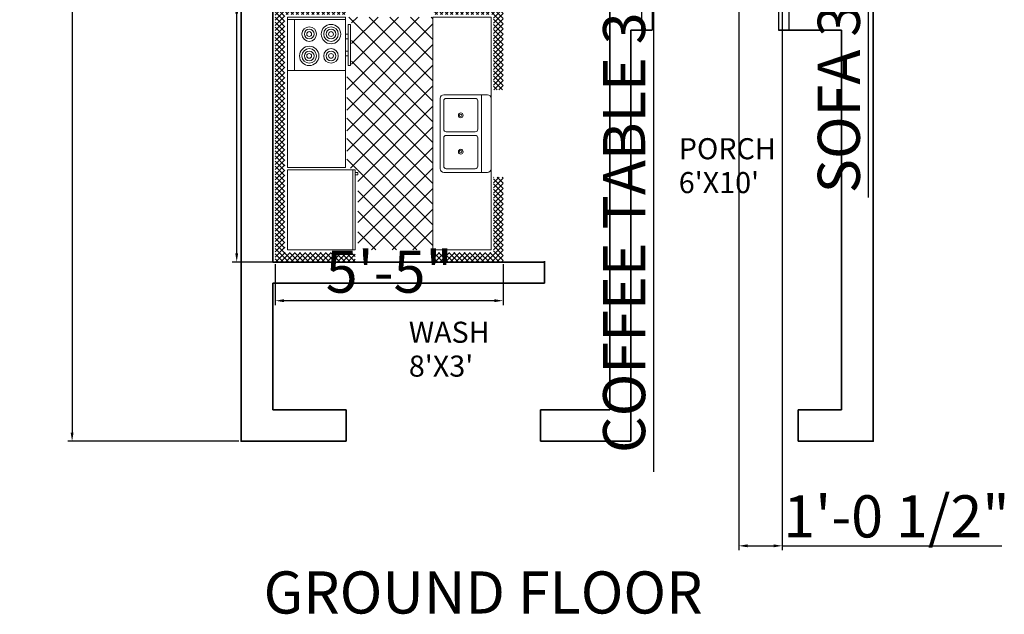
# Model space of a CAD drawing. Units: inches. Extents: x 2353 to 2961, y 642 to 1248.
# Tile 1 of 5: x 2353 to 2633, y 671 to 840. Entities that reach past the tile are written whole.
import ezdxf

# ---------------------------------------------------------------- set-up
doc = ezdxf.new("R2010")
doc.units = ezdxf.units.IN
for name, color, linetype, lineweight in [('A-ANNO-DIMS', 2, 'Continuous', 18), ('A-ANNO-TEXT', 7, 'Continuous', 25), ('A-AREA-IDEN', 7, 'Continuous', 18), ('A-DOOR', 4, 'Continuous', 25), ('A-FLOR-FIXT', 9, 'Continuous', 18), ('A-WALL', 7, 'Continuous', 35)]:
    doc.layers.add(name, color=color, linetype=linetype, lineweight=lineweight)
doc.styles.get("Standard").update_dxf_attribs({"font": 'arial.ttf'})
doc.dimstyles.new('ISO-25', dxfattribs={"dimtxt": 12, "dimasz": 2.5, "dimexe": 1.25, "dimexo": 0.625, "dimtad": 1, "dimdec": 1, "dimlunit": 3, "dimtxsty": 'Standard', "dimcen": 2.5, "dimadec": 0, "dimazin": 0, "dimtfac": 1, "dimtdec": 1, "dimtmove": 0, "dimatfit": 3, "dimfxl": 1, "dimarcsym": 0})

# ---------------------------------------------------------------- blocks, each defined once
blk = doc.blocks.new('Kitchen Layout - 7 x 8 ft')
for p, q in [((-5, 81.32), (2.68, 89)), ((-5, 83.44), (0.56, 89)), ((-5, 85.56), (-1.56, 89)), ((-5, 87.68), (-3.68, 89)), ((-1, 84.97), (-5, 88.97)), ((-1, 82.85), (-5, 86.85)), ((1.09, 85), (-2.91, 89)), ((3.21, 85), (-0.79, 89)), ((0.81, 85), (4.81, 89)), ((5.34, 85), (1.34, 89)), ((2.93, 85), (6.93, 89)), ((7.46, 85), (3.46, 89)), ((5.05, 85), (9.05, 89)), ((9.58, 85), (5.58, 89)), ((7.17, 85), (11.17, 89)), ((11.7, 85), (7.7, 89)), ((9.29, 85), (13.29, 89)), ((13.82, 85), (9.82, 89)), ((11.41, 85), (15.41, 89)), ((15.94, 85), (11.94, 89)), ((13.53, 85), (17.53, 89)), ((18.06, 85), (14.06, 89)), ((15.65, 85), (19.65, 89)), ((20.18, 85), (16.18, 89)), ((17.78, 85), (21.78, 89)), ((22.31, 85), (18.31, 89)), ((19.9, 85), (23.9, 89)), ((24.43, 85), (20.43, 89)), ((22.02, 85), (26.02, 89)), ((26.55, 85), (22.55, 89)), ((24.14, 85), (28.14, 89)), ((28.67, 85), (24.67, 89)), ((26.26, 85), (30.26, 89)), ((30.79, 85), (26.79, 89)), ((28.38, 85), (32.38, 89)), ((32.91, 85), (28.91, 89)), ((30.5, 85), (34.5, 89)), ((35.03, 85), (31.03, 89)), ((32.63, 85), (36.63, 89)), ((37.16, 85), (33.16, 89)), ((34.75, 85), (38.75, 89)), ((39.28, 85), (35.28, 89)), ((36.87, 85), (40.87, 89)), ((41.4, 85), (37.4, 89)), ((38.99, 85), (42.99, 89)), ((43.52, 85), (39.52, 89)), ((41.11, 85), (45.11, 89)), ((45.64, 85), (41.64, 89)), ((43.23, 85), (47.23, 89)), ((47.76, 85), (43.76, 89)), ((45.35, 85), (49.35, 89)), ((49.88, 85), (45.88, 89)), ((47.47, 85), (51.47, 89)), ((52, 85), (48, 89)), ((49.6, 85), (53.6, 89)), ((54.13, 85), (50.13, 89)), ((51.72, 85), (55.72, 89)), ((56.25, 85), (52.25, 89)), ((53.84, 85), (57.84, 89)), ((58.37, 85), (54.37, 89)), ((55.96, 85), (59.96, 89)), ((60.49, 85), (56.49, 89)), ((58.08, 85), (62.08, 89)), ((62.61, 85), (58.61, 89)), ((60.2, 85), (64.2, 89)), ((64.73, 85), (60.73, 89)), ((62.32, 85), (66.32, 89)), ((66.85, 85), (62.85, 89)), ((64.45, 85), (68.45, 89)), ((68.97, 85), (64.97, 89)), ((66.57, 85), (70.57, 89)), ((71.1, 85), (67.1, 89)), ((68.69, 85), (72.69, 89)), ((73.22, 85), (69.22, 89)), ((70.81, 85), (74.81, 89)), ((75.34, 85), (71.34, 89)), ((72.93, 85), (76.93, 89)), ((77.46, 85), (73.46, 89)), ((75.05, 85), (79.05, 89)), ((79.58, 85), (75.58, 89)), ((77.17, 85), (81.17, 89)), ((81.7, 85), (77.7, 89)), ((79.29, 85), (83.29, 89)), ((83.82, 85), (79.82, 89)), ((81.42, 85), (85.42, 89)), ((85.95, 85), (81.95, 89)), ((83.54, 85), (87.54, 89)), ((88.07, 85), (84.07, 89)), ((85.66, 85), (89.66, 89)), ((90.19, 85), (86.19, 89)), ((87.78, 85), (91.78, 89)), ((92.31, 85), (88.31, 89)), ((89.9, 85), (93.9, 89)), ((94.43, 85), (90.43, 89)), ((92.02, 85), (96.02, 89)), ((96.55, 85), (92.55, 89)), ((94.14, 85), (98.14, 89)), ((101, 82.67), (94.67, 89)), ((96.27, 85), (100.27, 89)), ((101, 84.79), (96.79, 89)), ((97, 83.61), (101, 87.61)), ((97, 81.49), (101, 85.49)), ((101, 86.92), (98.92, 89)), ((-1, 80.73), (-5, 84.73)), ((-5, 79.19), (-1, 83.19)), ((-1, 78.61), (-5, 82.61)), ((34, 84), (96, 84)), ((34, 60), (34, 84)), ((96, 84), (96, 60)), ((101, 80.55), (97, 84.55)), ((97, 79.37), (101, 83.37)), ((101, 78.43), (97, 82.43)), ((97, 77.25), (101, 81.25)), ((-5, 77.07), (-1, 81.07)), ((-1, 76.49), (-5, 80.49)), ((-5, 74.95), (-1, 78.95)), ((-1, 74.36), (-5, 78.36)), ((74, 81), (95, 81)), ((101, 76.31), (97, 80.31)), ((97, 75.13), (101, 79.13)), ((101, 74.19), (97, 78.19)), ((-5, 72.83), (-1, 76.83)), ((-1, 72.24), (-5, 76.24)), ((-5, 70.71), (-1, 74.71)), ((-1, 70.12), (-5, 74.12)), ((97, 73.01), (101, 77.01)), ((101, 72.07), (97, 76.07)), ((97, 70.89), (101, 74.89)), ((101, 69.95), (97, 73.95)), ((-5, 68.59), (-1, 72.59)), ((-1, 68), (-5, 72)), ((-5, 66.47), (-1, 70.47)), ((-1, 65.88), (-5, 69.88)), ((97, 68.76), (101, 72.76)), ((101, 67.82), (97, 71.82)), ((97, 66.64), (101, 70.64)), ((101, 65.7), (97, 69.7)), ((-5, 64.35), (-1, 68.35)), ((-1, 63.76), (-5, 67.76)), ((-5, 62.22), (-1, 66.22)), ((-1, 61.64), (-5, 65.64)), ((97, 64.52), (101, 68.52)), ((101, 63.58), (97, 67.58)), ((97, 62.4), (101, 66.4)), ((101, 61.46), (97, 65.46)), ((-5, 60.1), (-1, 64.1)), ((-1, 59.52), (-5, 63.52)), ((-5, 57.98), (-1, 61.98)), ((-1, 57.39), (-5, 61.39)), ((97, 60.28), (101, 64.28)), ((100.34, 60), (97, 63.34)), ((98.22, 60), (97, 61.22)), ((98.84, 60), (101, 62.16)), ((-1.73, 56), (-5, 59.27)), ((-3.85, 56), (-5, 57.15)), ((-4.86, 56), (-1, 59.86)), ((-2.74, 56), (-1, 57.74)), ((0, 57), (33, 57)), ((10.4, 24), (45.9, 59.5)), ((18.88, 24), (54.38, 59.5)), ((27.37, 24), (62.87, 59.5)), ((33.03, 55.11), (37.41, 59.5)), ((67.71, 24), (33.68, 58.04)), ((96, 60), (34, 60)), ((35.85, 24), (71.35, 59.5)), ((76.2, 24), (40.7, 59.5)), ((44.34, 24), (77.84, 57.5)), ((84.68, 24), (49.18, 59.5)), ((52.82, 24), (86.32, 57.5)), ((93.17, 24), (57.67, 59.5)), ((61.31, 24), (96, 58.69)), ((96, 29.65), (66.15, 59.5)), ((96, 38.14), (76.64, 57.5)), ((80, 60), (80, 59)), ((82, 59), (82, 60)), ((96, 46.63), (85.13, 57.5)), ((87, 59), (87, 60)), ((89, 60), (89, 59)), ((96, 55.11), (93.57, 57.54)), ((100.96, 60), (101, 60.04)), ((0, 30.57), (24.43, 55)), ((0, 39.06), (15.94, 55)), ((0, 47.54), (7.46, 55)), ((1.91, 24), (32.91, 55)), ((33.77, 24), (2.77, 55)), ((42.26, 24), (11.26, 55)), ((50.74, 24), (19.74, 55)), ((59.23, 24), (28.23, 55)), ((31, 55), (31, 56)), ((32, 55), (31, 55)), ((32, 56), (32, 55)), ((25.29, 24), (0, 49.29)), ((69.79, 24), (96, 50.21)), ((16.8, 24), (0, 40.8)), ((78.28, 24), (96, 41.72)), ((86.76, 24), (96, 33.24)), ((8.32, 24), (0, 32.32)), ((95.25, 24), (96, 24.75)), ((-5, 21.92), (-2.92, 24)), ((-5, 19.8), (-1, 23.8)), ((-1, 19.21), (-5, 23.21)), ((-5, 17.68), (-1, 21.68)), ((-1, 17.09), (-5, 21.09)), ((-1, 21.33), (-3.67, 24)), ((-1, 23.45), (-1.55, 24)), ((0, 24), (96, 24)), ((0, 0), (0, 24)), ((96, 24), (96, 0)), ((97, 22.1), (98.9, 24)), ((97, 19.97), (101, 23.97)), ((101, 19.03), (97, 23.03)), ((97, 17.85), (101, 21.85)), ((101, 16.91), (97, 20.91)), ((101, 21.16), (98.16, 24)), ((101, 23.28), (100.28, 24)), ((-5, 15.55), (-1, 19.55)), ((-1, 14.97), (-5, 18.97)), ((-5, 13.43), (-1, 17.43)), ((-1, 12.85), (-5, 16.85)), ((47.25, 6.5), (47.25, 18.5)), ((48.75, 18.5), (48.75, 6.5)), ((97, 15.73), (101, 19.73)), ((101, 14.79), (97, 18.79)), ((97, 13.61), (101, 17.61)), ((101, 12.67), (97, 16.67)), ((-5, 11.31), (-1, 15.31)), ((-1, 10.73), (-5, 14.73)), ((-5, 9.19), (-1, 13.19)), ((-1, 8.6), (-5, 12.6)), ((97, 11.49), (101, 15.49)), ((101, 10.55), (97, 14.55)), ((97, 9.37), (101, 13.37)), ((101, 8.43), (97, 12.43)), ((-5, 7.07), (-1, 11.07)), ((-1, 6.48), (-5, 10.48)), ((-5, 4.95), (-1, 8.95)), ((-1, 4.36), (-5, 8.36)), ((97, 7.25), (101, 11.25)), ((101, 6.31), (97, 10.31)), ((97, 5.12), (101, 9.12)), ((101, 4.18), (97, 8.18)), ((-5, 2.83), (-1, 6.83)), ((-1, 2.24), (-5, 6.24)), ((-5, 0.71), (-1, 4.71)), ((-1, 0.12), (-5, 4.12)), ((97, 3), (101, 7)), ((101, 2.06), (97, 6.06)), ((97, 0.88), (101, 4.88)), ((-5, -1.42), (-1, 2.58)), ((2, -5), (-5, 2)), ((-5, -3.54), (-1, 0.46)), ((96, 0), (0, 0)), ((64, 4), (32, 4)), ((93.24, -5), (101, 2.76)), ((95.36, -5), (101, 0.64)), ((101, -0.06), (97, 3.94)), ((101, -2.18), (97, 1.82)), ((-0.12, -5), (-5, -0.12)), ((-2.25, -5), (-5, -2.25)), ((-4.34, -5), (-0.34, -1)), ((-2.22, -5), (1.78, -1)), ((-0.1, -5), (3.9, -1)), ((4.12, -5), (0.12, -1)), ((2.02, -5), (6.02, -1)), ((6.24, -5), (2.24, -1)), ((4.14, -5), (8.14, -1)), ((8.36, -5), (4.36, -1)), ((6.27, -5), (10.27, -1)), ((10.48, -5), (6.48, -1)), ((8.39, -5), (12.39, -1)), ((12.6, -5), (8.6, -1)), ((10.51, -5), (14.51, -1)), ((14.73, -5), (10.73, -1)), ((12.63, -5), (16.63, -1)), ((16.85, -5), (12.85, -1)), ((14.75, -5), (18.75, -1)), ((18.97, -5), (14.97, -1)), ((16.87, -5), (20.87, -1)), ((21.09, -5), (17.09, -1)), ((18.99, -5), (22.99, -1)), ((23.21, -5), (19.21, -1)), ((21.11, -5), (25.11, -1)), ((25.33, -5), (21.33, -1)), ((23.24, -5), (27.24, -1)), ((27.45, -5), (23.45, -1)), ((25.36, -5), (29.36, -1)), ((29.57, -5), (25.57, -1)), ((27.48, -5), (30, -2.48)), ((30, -3.3), (27.7, -1)), ((30, -1.18), (29.82, -1)), ((66, -2.54), (67.54, -1)), ((66, -4.66), (69.66, -1)), ((69.88, -5), (66, -1.12)), ((67.76, -5), (66, -3.24)), ((67.78, -5), (71.78, -1)), ((72, -5), (68, -1)), ((69.9, -5), (73.9, -1)), ((74.12, -5), (70.12, -1)), ((72.03, -5), (76.03, -1)), ((76.24, -5), (72.24, -1)), ((74.15, -5), (78.15, -1)), ((78.36, -5), (74.36, -1)), ((76.27, -5), (80.27, -1)), ((80.49, -5), (76.49, -1)), ((78.39, -5), (82.39, -1)), ((82.61, -5), (78.61, -1)), ((80.51, -5), (84.51, -1)), ((84.73, -5), (80.73, -1)), ((82.63, -5), (86.63, -1)), ((86.85, -5), (82.85, -1)), ((84.75, -5), (88.75, -1)), ((88.97, -5), (84.97, -1)), ((86.88, -5), (90.88, -1)), ((91.09, -5), (87.09, -1)), ((89, -5), (93, -1)), ((93.21, -5), (89.21, -1)), ((91.12, -5), (95.12, -1)), ((95.34, -5), (91.34, -1)), ((97.46, -5), (93.46, -1)), ((99.58, -5), (95.58, -1)), ((101, -4.3), (97, -0.3)), ((97.48, -5), (101, -1.48)), ((99.6, -5), (101, -3.6)), ((-4.37, -5), (-5, -4.37)), ((29.6, -5), (30, -4.6))]:
    blk.add_line(p, q)
for points in [[(0, 56), (0, 84), (33, 84), (33, 56)], [(74, 60), (74, 84), (95, 84), (95, 60)], [(76, 58), (76, 59), (93, 59), (93, 58)]]:
    blk.add_lwpolyline(points, close=True)
for points in [[(33.5, 21), (62.5, 21)], [(32, 1.5), (32, 19.5)], [(33.5, 6.5), (33.5, 18.5)], [(34.5, 19.5), (46.25, 19.5)], [(49.75, 19.5), (61.5, 19.5)], [(62.5, 18.5), (62.5, 6.5)], [(64, 19.5), (64, 1.5)], [(46.25, 5.5), (34.5, 5.5)], [(61.5, 5.5), (49.75, 5.5)], [(62.5, 0), (33.5, 0)]]:
    blk.add_lwpolyline(points)
for centre, radius in [((80, 75), 4), ((80, 75), 3), ((89, 75), 3), ((80, 75), 2), ((80, 75), 1), ((89, 75), 2), ((89, 75), 1), ((89, 66), 4), ((80, 66), 3), ((80, 66), 2), ((80, 66), 1), ((89, 66), 3), ((89, 66), 2), ((89, 66), 1), ((40.5, 12.5), 1), ((40.5, 12.5), 0.5), ((55.5, 12.5), 1), ((55.5, 12.5), 0.5)]:
    blk.add_circle(centre, radius)
for centre, radius, start, end in [((33.5, 19.5), 1.5, 90, 180), ((62.5, 19.5), 1.5, 0, 90), ((34.5, 18.5), 1, 90, 180), ((46.25, 18.5), 1, 0, 90), ((49.75, 18.5), 1, 90, 180), ((61.5, 18.5), 1, 0, 90), ((34.5, 6.5), 1, 180, 270), ((46.25, 6.5), 1, 270, 0), ((49.75, 6.5), 1, 180, 270), ((61.5, 6.5), 1, 270, 0), ((33.5, 1.5), 1.5, 180, 270), ((62.5, 1.5), 1.5, 270, 0)]:
    blk.add_arc(centre, radius, start, end)
blk = doc.blocks.new('*D8')
at = {"layer": 'A-ANNO-DIMS', "color": 0, "lineweight": -2, "transparency": 16777216}
for p, q in [((2415.1, 1200.48), (2366.34, 1200.48)), ((2367.59, 1197.98), (2367.59, 722.98)), ((2415.1, 720.48), (2366.34, 720.48))]:
    blk.add_line(p, q, dxfattribs=at)
at = {"layer": 'A-ANNO-DIMS', "color": 0, "transparency": 16777216}
for points in [[(2367.17, 1197.98), (2368.01, 1197.98), (2367.59, 1200.48)], [(2367.17, 722.98), (2368.01, 722.98), (2367.59, 720.48)]]:
    blk.add_solid(points, dxfattribs=at)
at = {"layer": 'Defpoints', "color": 0, "transparency": 16777216}
for p in [(2415.72, 1200.48), (2367.59, 720.48), (2415.72, 720.48)]:
    blk.add_point(p, dxfattribs=at)
at = {"layer": 'A-ANNO-DIMS', "color": 0, "transparency": 16777216, "insert": (2360.84, 960.48), "char_height": 12, "attachment_point": 5, "rotation": 90}
blk.add_mtext("40'", dxfattribs=at)
blk = doc.blocks.new('DOOR-SINGLE-36IN')
for p, q in [((0, 6), (0, 0)), ((3, 6), (3, 0)), ((39, 6), (39, 0)), ((42, 6), (42, 0))]:
    blk.add_line(p, q)
blk.add_lwpolyline([(3, 6), (6, 6), (6, 42), (3, 42)], close=True)
blk.add_arc((4.5, 7.5), 34.53, 357.5104, 92.4896)
blk = doc.blocks.new('*D25')
at = {"layer": 'A-ANNO-DIMS', "color": 0, "lineweight": -2, "transparency": 16777216}
for p, q in [((2538.14, 943.02), (2531.92, 943.02)), ((2533.17, 940.52), (2533.17, 908.21)), ((2538.14, 905.71), (2531.92, 905.71)), ((2533.17, 905.71), (2533.17, 711.83))]:
    blk.add_line(p, q, dxfattribs=at)
at = {"layer": 'A-ANNO-DIMS', "color": 0, "transparency": 16777216}
for points in [[(2532.75, 940.52), (2533.58, 940.52), (2533.17, 943.02)], [(2532.75, 908.21), (2533.58, 908.21), (2533.17, 905.71)]]:
    blk.add_solid(points, dxfattribs=at)
at = {"layer": 'Defpoints', "color": 0, "transparency": 16777216}
for p in [(2538.76, 943.02), (2533.17, 905.71), (2538.76, 905.71)]:
    blk.add_point(p, dxfattribs=at)
at = {"layer": 'A-ANNO-DIMS', "color": 0, "transparency": 16777216, "insert": (2526.33, 807.52), "char_height": 12, "attachment_point": 5, "rotation": 90}
blk.add_mtext('COFFEE TABLE 3\'-1 1/2"', dxfattribs=at)
blk = doc.blocks.new('*D29')
at = {"layer": 'A-ANNO-DIMS', "color": 0, "lineweight": -2, "transparency": 16777216}
for p, q in [((2588.67, 945.47), (2595.56, 945.47)), ((2594.31, 942.97), (2594.31, 906.24)), ((2588.67, 903.74), (2595.56, 903.74)), ((2594.31, 903.74), (2594.31, 789.88))]:
    blk.add_line(p, q, dxfattribs=at)
at = {"layer": 'A-ANNO-DIMS', "color": 0, "transparency": 16777216}
for points in [[(2593.89, 942.97), (2594.72, 942.97), (2594.31, 945.47)], [(2593.89, 906.24), (2594.72, 906.24), (2594.31, 903.74)]]:
    blk.add_solid(points, dxfattribs=at)
at = {"layer": 'Defpoints', "color": 0, "transparency": 16777216}
for p in [(2588.05, 945.47), (2588.05, 903.74), (2594.31, 903.74)]:
    blk.add_point(p, dxfattribs=at)
at = {"layer": 'A-ANNO-DIMS', "color": 0, "transparency": 16777216, "insert": (2587.47, 845.56), "char_height": 12, "attachment_point": 5, "rotation": 90}
blk.add_mtext('SOFA 3\'-5 1/2"', dxfattribs=at)
blk = doc.blocks.new('*D31')
at = {"layer": 'A-ANNO-DIMS', "color": 0, "lineweight": -2, "transparency": 16777216}
for p, q in [((2414.46, 844.67), (2414.46, 1001.8)), ((2424.82, 844.67), (2413.21, 844.67)), ((2414.46, 773.98), (2414.46, 842.17)), ((2424.82, 771.48), (2413.21, 771.48))]:
    blk.add_line(p, q, dxfattribs=at)
at = {"layer": 'A-ANNO-DIMS', "color": 0, "transparency": 16777216}
for points in [[(2414.05, 842.17), (2414.88, 842.17), (2414.46, 844.67)], [(2414.05, 773.98), (2414.88, 773.98), (2414.46, 771.48)]]:
    blk.add_solid(points, dxfattribs=at)
at = {"layer": 'Defpoints', "color": 0, "transparency": 16777216}
for p in [(2414.46, 844.67), (2425.44, 844.67), (2425.44, 771.48)]:
    blk.add_point(p, dxfattribs=at)
at = {"layer": 'A-ANNO-DIMS', "color": 0, "transparency": 16777216, "insert": (2407.63, 924.49), "char_height": 12, "attachment_point": 5, "rotation": 90}
blk.add_mtext('KITCHEN UNIT 6\'-1"', dxfattribs=at)
blk = doc.blocks.new('*D32')
at = {"layer": 'A-ANNO-DIMS', "color": 0, "lineweight": -2, "transparency": 16777216}
for p, q in [((2425.44, 770.86), (2425.44, 759.25)), ((2490.35, 770.86), (2490.35, 759.25)), ((2487.85, 760.5), (2427.94, 760.5))]:
    blk.add_line(p, q, dxfattribs=at)
at = {"layer": 'A-ANNO-DIMS', "color": 0, "transparency": 16777216}
for points in [[(2427.94, 760.92), (2427.94, 760.09), (2425.44, 760.5)], [(2487.85, 760.92), (2487.85, 760.09), (2490.35, 760.5)]]:
    blk.add_solid(points, dxfattribs=at)
at = {"layer": 'Defpoints', "color": 0, "transparency": 16777216}
for p in [(2425.44, 771.48), (2490.35, 771.48), (2425.44, 760.5)]:
    blk.add_point(p, dxfattribs=at)
at = {"layer": 'A-ANNO-DIMS', "color": 0, "transparency": 16777216, "insert": (2457.89, 767.23), "char_height": 12, "attachment_point": 5}
blk.add_mtext('5\'-5"', dxfattribs=at)
blk = doc.blocks.new('*D40')
at = {"layer": 'A-ANNO-DIMS', "color": 0, "lineweight": -2, "transparency": 16777216}
for p, q in [((2557.42, 905.09), (2557.42, 689.48)), ((2569.83, 903.11), (2569.83, 689.48)), ((2559.92, 690.73), (2567.33, 690.73)), ((2569.83, 690.73), (2632.31, 690.73))]:
    blk.add_line(p, q, dxfattribs=at)
at = {"layer": 'A-ANNO-DIMS', "color": 0, "transparency": 16777216}
for points in [[(2559.92, 691.15), (2559.92, 690.32), (2557.42, 690.73)], [(2567.33, 691.15), (2567.33, 690.32), (2569.83, 690.73)]]:
    blk.add_solid(points, dxfattribs=at)
at = {"layer": 'Defpoints', "color": 0, "transparency": 16777216}
for p in [(2557.42, 905.71), (2569.83, 903.74), (2569.83, 690.73)]:
    blk.add_point(p, dxfattribs=at)
at = {"layer": 'A-ANNO-DIMS', "color": 0, "transparency": 16777216, "insert": (2602.32, 697.56), "char_height": 12, "attachment_point": 5}
blk.add_mtext('1\'-0 1/2"', dxfattribs=at)

msp = doc.modelspace()

# ---------------------------------------------------------------- linework, layer by layer
at = {"layer": 'A-WALL'}
for p, q in [((2424.72, 873.48), (2424.72, 771.48)), ((2520.72, 873.48), (2520.72, 729.48)), ((2526.72, 837.48), (2532.72, 837.48)), ((2526.72, 837.48), (2526.72, 729.48)), ((2568.72, 837.48), (2586.72, 837.48)), ((2586.72, 729.48), (2586.72, 837.48)), ((2424.72, 771.48), (2502.15, 771.48)), ((2502.15, 771.74), (2502.15, 765.48)), ((2424.72, 765.48), (2502.15, 765.48)), ((2424.72, 765.48), (2424.72, 729.48)), ((2520.72, 765.48), (2520.72, 729.48)), ((2424.72, 729.48), (2445.67, 729.48)), ((2445.67, 729.48), (2445.67, 720.48)), ((2500.97, 729.48), (2500.97, 720.48)), ((2500.97, 729.48), (2520.72, 729.48)), ((2526.72, 729.48), (2526.72, 720.48)), ((2574.3, 729.48), (2586.72, 729.48)), ((2574.3, 729.48), (2574.3, 720.48))]:
    msp.add_line(p, q, dxfattribs=at)
for points in [[(2574.3, 720.48), (2595.72, 720.48), (2595.72, 1200.48), (2415.72, 1200.48), (2415.72, 720.48), (2445.67, 720.48)], [(2500.97, 720.48), (2526.72, 720.48)]]:
    msp.add_lwpolyline(points, dxfattribs=at)

# ---------------------------------------------------------------- block references
at = {"layer": 'A-DOOR'}
msp.add_blockref('DOOR-SINGLE-36IN', (2529.72, 837.48), dxfattribs=at)
at = {"layer": 'A-FLOR-FIXT', "xscale": 0.690484494816598, "yscale": 0.690484494816598, "zscale": 0.690484494816598, "rotation": 90}
msp.add_blockref('Kitchen Layout - 7 x 8 ft', (2486.89, 774.94), dxfattribs=at)

# ---------------------------------------------------------------- texts
at = {"layer": 'A-ANNO-TEXT'}
msp.add_text('GROUND FLOOR', height=12, dxfattribs=at).set_placement((2422.11, 671.46))
at = {"layer": 'A-AREA-IDEN'}
for s, p in [('PORCH', (2540.34, 800.76)), ("6'X10'", (2540.34, 791.12)), ('WASH', (2463.48, 748.52)), ("8'X3'", (2463.48, 738.88))]:
    msp.add_text(s, height=6, dxfattribs=at).set_placement(p)

# ---------------------------------------------------------------- dimensions: what is measured, and where the dimension line sits
at = {"layer": 'A-ANNO-DIMS'}
for base, p1, p2, angle, override, picture, middle in [((2367.59, 720.48), (2415.72, 1200.48), (2415.72, 720.48), 90, {"dimclrd": 0, "dimclre": 0, "dimclrt": 0}, '*D8', (2360.84, 960.48)), ((2425.44, 760.5), (2490.35, 771.48), (2425.44, 771.48), 180, {"dimdec": 1, "dimlfac": 1, "dimrnd": 0, "dimzin": 1, "dimdsep": 46, "dimlunit": 4, "dimfrac": 2}, '*D32', (2457.89, 767.23))]:
    dim = msp.add_linear_dim(base=base, p1=p1, p2=p2, angle=angle, dimstyle='ISO-25', override=override, dxfattribs=at)
    dim.commit()
    dim.dimension.update_dxf_attribs({"geometry": picture, "text_midpoint": middle})
for base, p1, p2, angle, text, picture, middle in [((2414.46, 844.67), (2425.44, 771.48), (2425.44, 844.67), 90, 'KITCHEN UNIT <>', '*D31', (2407.63, 924.49)), ((2594.31, 903.74), (2588.05, 945.47), (2588.05, 903.74), 270, 'SOFA <>', '*D29', (2587.47, 845.56)), ((2533.17, 905.71), (2538.76, 943.02), (2538.76, 905.71), 270, 'COFFEE TABLE <>', '*D25', (2526.33, 807.52))]:
    dim = msp.add_linear_dim(base=base, p1=p1, p2=p2, angle=angle, text=text, dimstyle='ISO-25', override={"dimdec": 1, "dimlfac": 1, "dimrnd": 0, "dimzin": 1, "dimdsep": 46, "dimlunit": 4, "dimfrac": 2}, dxfattribs=at)
    dim.commit()
    dim.dimension.update_dxf_attribs({"geometry": picture, "text_midpoint": middle})
dim = msp.add_linear_dim(base=(2569.83, 690.73), p1=(2557.42, 905.71), p2=(2569.83, 903.74), dimstyle='ISO-25', override={"dimdec": 1, "dimlfac": 1, "dimrnd": 0, "dimzin": 1, "dimdsep": 46, "dimlunit": 4, "dimfrac": 2}, dxfattribs=at)
dim.commit()
dim.dimension.update_dxf_attribs({"geometry": '*D40', "text_midpoint": (2602.32, 697.56)})

doc.saveas('drawing.dxf')
